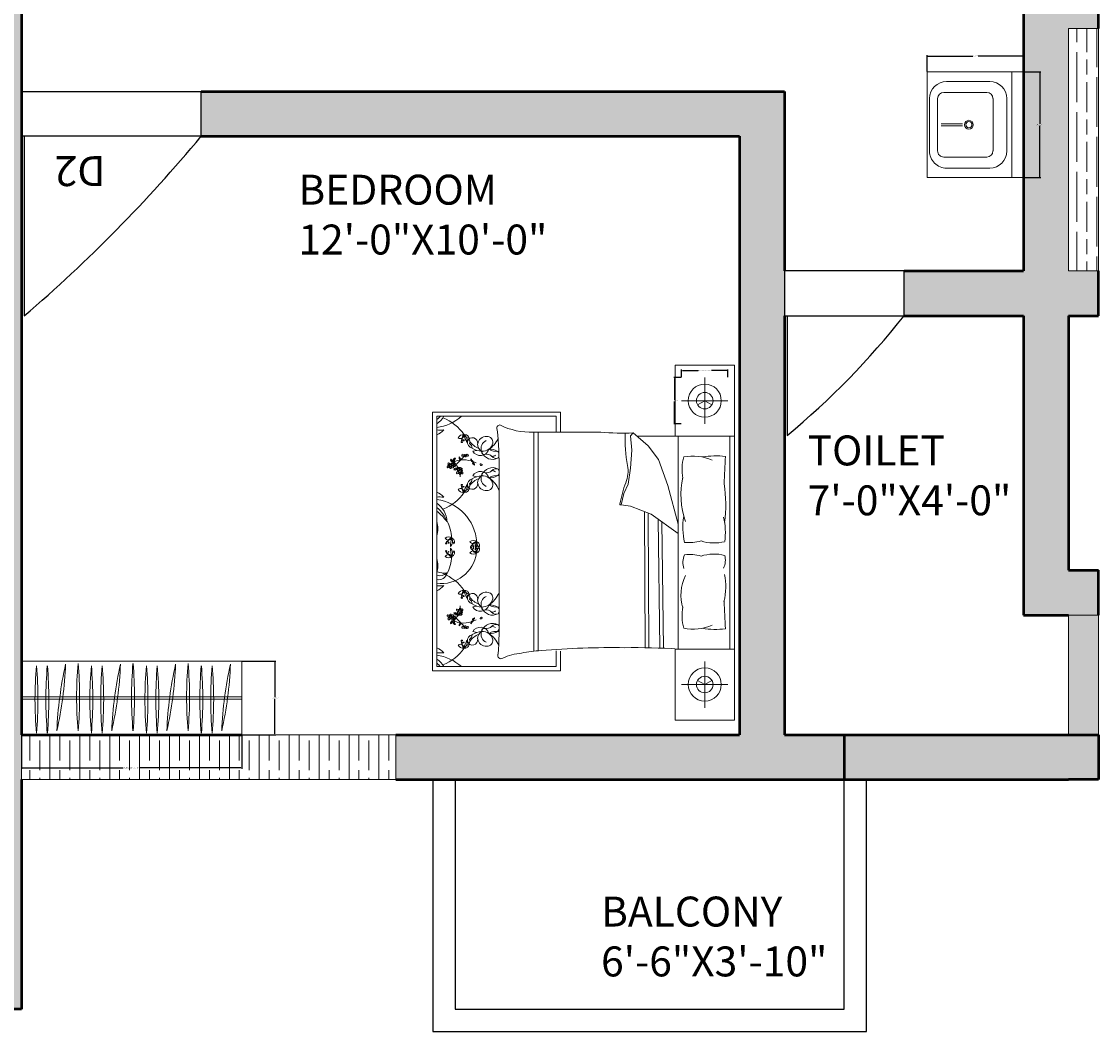
# Model space of a CAD drawing. Units: inches. Extents: x -12 to 604, y -566 to 58.
# Tile 3 of 12: x 388 to 604, y -534 to -332. Entities that reach past the tile are written whole.
import ezdxf

# ---------------------------------------------------------------- set-up
doc = ezdxf.new("R2010")
doc.units = ezdxf.units.IN
doc.header["$MEASUREMENT"] = 0
for name, color, linetype, lineweight in [('A-ANNO-DIMS', 2, 'Continuous', 18), ('A-ANNO-TEXT', 7, 'Continuous', 18), ('A-AREA-IDEN', 7, 'Continuous', 18), ('A-DOOR', 4, 'Continuous', 25), ('A-FLOR-FIXT', 9, 'Continuous', 18), ('A-FLOR-RAIL', 7, 'Continuous', 25), ('A-FURN', 8, 'Continuous', 18), ('A-GLAZ', 82, 'Continuous', 18), ('A-GLAZ-PATT', 82, 'Continuous', 13), ('A-WALL', 7, 'Continuous', 50), ('A-WALL-PATT', 18, 'Continuous', 13)]:
    doc.layers.add(name, color=color, linetype=linetype, lineweight=lineweight)
doc.styles.get("Standard").update_dxf_attribs({"font": 'arial.ttf'})
doc.dimstyles.get("Standard").update_dxf_attribs({"dimtxt": 0.18, "dimasz": 0.18, "dimexe": 0.18, "dimexo": 0.0625, "dimgap": 0.09, "dimtad": 0, "dimtih": 1, "dimtoh": 1, "dimdec": 0, "dimzin": 0, "dimdsep": 46, "dimlunit": 3, "dimtxsty": 'Standard', "dimcen": 0.09, "dimadec": 0, "dimazin": 0, "dimtfac": 1, "dimtdec": 0, "dimtofl": 0, "dimtmove": 0, "dimatfit": 3, "dimfxl": 1, "dimtolj": 1, "dimtzin": 0, "dimarcsym": 0})
pattern_1 = [(90, (0, 0), (6, -4e-16), [10, -2]), (90, (2, -2), (6, -4e-16), [6, -1.5, 3, -1.5]), (90, (4, -5), (6, -4e-16), [10, -2])]

# ---------------------------------------------------------------- blocks, each defined once
blk = doc.blocks.new('М14 600х655')
for p, q in [((-655, 600), (-655, 0)), ((-655, 600), (-655, 0)), ((-655, 0), (-655, 600)), ((0, 600), (-655, 600)), ((0, 0), (0, 600)), ((0, 525), (-655, 525)), ((-165.1, 494.1), (-489.9, 494.1)), ((-165.4, 408.4), (-490.2, 408.4)), ((-595.8, 388.1), (-595.8, 121.3)), ((-528.4, 370.1), (-528.4, 103.3)), ((-127.2, 103.3), (-127.2, 370.1)), ((-59.2, 121.3), (-59.2, 388.1)), ((-333.5, 87.1), (-333.5, 219.6)), ((-321.5, 87.1), (-321.5, 219.6)), ((-655, 0), (-655, 0)), ((-655, 0), (-655, 0)), ((-655, 0), (0, 0)), ((-655, 0), (0, 0)), ((-490.2, 65.1), (-165.4, 65.1)), ((-489.9, 15.4), (-165.1, 15.4))]:
    blk.add_line(p, q)
for radius in [27.6, 19.3]:
    blk.add_circle((-327.5, 258.9), radius)
for centre, radius, start, end in [((-489.9, 388.1), 105.9, 90, 180), ((-165.1, 388.1), 105.9, 0, 90), ((-490.2, 370.1), 38.2, 90, 180), ((-165.4, 370.1), 38.2, 0, 90), ((-489.9, 121.3), 105.9, 180, 270), ((-490.2, 103.3), 38.2, 180, 270), ((-165.4, 103.3), 38.2, 270, 0), ((-165.1, 121.3), 105.9, 270, 0)]:
    blk.add_arc(centre, radius, start, end)
blk = doc.blocks.new('WARDROBE-HANGING-RAIL')
for p, q in [((44.18, 14.73), (0, 14.73)), ((0, 14.73), (0, 0)), ((44.18, 14.73), (44.18, 0)), ((44.18, 7.61), (0, 7.61)), ((44.18, 7.12), (0, 7.12)), ((44.18, 0), (0, 0))]:
    blk.add_line(p, q)
for centre, start, end in [((80.19, 7.07), 175.0028, 184.9972), ((-74.2, 7.07), 355.0028, 4.9972), ((82.37, 7.07), 175.0028, 184.9972), ((-72.01, 7.07), 355.0028, 4.9972), ((-68.57, 17.55), 347.508, 357.5023), ((84.5, -2.59), 167.508, 177.5023), ((88.54, 7.54), 175.0028, 184.9972), ((-65.84, 7.54), 355.0028, 4.9972), ((91.2, 7.07), 175.0028, 184.9972), ((-63.19, 7.07), 355.0028, 4.9972), ((93.38, 7.07), 175.0028, 184.9972), ((-61.01, 7.07), 355.0028, 4.9972), ((-57.56, 17.55), 347.508, 357.5023), ((95.51, -2.59), 167.508, 177.5023), ((99.55, 7.54), 175.0028, 184.9972), ((-54.83, 7.54), 355.0028, 4.9972), ((102.24, 7.07), 175.0028, 184.9972), ((-52.14, 7.07), 355.0028, 4.9972), ((104.43, 7.07), 175.0028, 184.9972), ((-49.96, 7.07), 355.0028, 4.9972), ((106.56, -2.59), 167.508, 177.5023), ((-46.51, 17.55), 347.508, 357.5023), ((110.6, 7.54), 175.0028, 184.9972), ((-43.79, 7.54), 355.0028, 4.9972), ((113.25, 7.07), 175.0028, 184.9972), ((-41.13, 7.07), 355.0028, 4.9972), ((115.43, 7.07), 175.0028, 184.9972), ((-38.95, 7.07), 355.0028, 4.9972), ((117.56, -2.59), 167.508, 177.5023), ((-35.5, 17.55), 347.508, 357.5023)]:
    blk.add_arc(centre, 77.49, start, end)
blk = doc.blocks.new('BALCONY-RAIL-U')
for p, q in [((0, 50.5), (0, 4.5)), ((4.5, 50.5), (4.5, 4.5)), ((82.5, 4.5), (82.5, 50.5)), ((87, 4.5), (87, 50.5)), ((0, 4.5), (0, 0)), ((4.5, 4.5), (82.5, 4.5)), ((87, 0), (87, 4.5)), ((0, 0), (4.5, 0)), ((4.5, 0), (82.5, 0)), ((82.5, 0), (87, 0))]:
    blk.add_line(p, q)
blk = doc.blocks.new('BEDSIDE-LAMP-169')
for p, q in [((4.65, 9.3), (4.65, 0)), ((0, 4.65), (9.3, 4.65))]:
    blk.add_line(p, q)
for points in [[(4.65, 4.65), (3.21, 5.48)], [(4.65, 4.65), (6.09, 5.48)]]:
    blk.add_lwpolyline(points)
for radius in [3.32, 1.66]:
    blk.add_circle((4.65, 4.65), radius)
blk = doc.blocks.new('*D21')
at = {"layer": 'A-ANNO-DIMS', "color": 0, "lineweight": -2, "transparency": 16777216}
for p, q in [((388.32, -474.92), (388.32, -481.67)), ((432.5, -474.92), (432.5, -481.67)), ((388.5, -481.49), (408.68, -481.49)), ((432.32, -481.49), (412.15, -481.49))]:
    blk.add_line(p, q, dxfattribs=at)
at = {"layer": 'A-ANNO-DIMS', "color": 0, "transparency": 16777216}
for points in [[(388.5, -481.46), (388.5, -481.52), (388.32, -481.49)], [(432.32, -481.46), (432.32, -481.52), (432.5, -481.49)]]:
    blk.add_solid(points, dxfattribs=at)
at = {"layer": 'Defpoints', "color": 0, "transparency": 16777216}
for p in [(388.32, -474.86), (432.5, -474.86), (432.5, -481.49)]:
    blk.add_point(p, dxfattribs=at)
at = {"layer": 'A-ANNO-DIMS', "color": 0, "transparency": 16777216, "insert": (410.41, -481.49), "char_height": 0.18, "attachment_point": 5}
blk.add_mtext('\\A1;WARDROBE RAIL 3\'-8" TYP.', dxfattribs=at)
blk = doc.blocks.new('*D22')
at = {"layer": 'A-ANNO-DIMS', "color": 0, "lineweight": -2, "transparency": 16777216}
for p, q in [((432.57, -460.13), (439.31, -460.13)), ((439.13, -460.31), (439.13, -467.31)), ((439.13, -474.68), (439.13, -467.68)), ((432.57, -474.86), (439.31, -474.86))]:
    blk.add_line(p, q, dxfattribs=at)
at = {"layer": 'A-ANNO-DIMS', "color": 0, "transparency": 16777216}
for points in [[(439.1, -460.31), (439.16, -460.31), (439.13, -460.13)], [(439.1, -474.68), (439.16, -474.68), (439.13, -474.86)]]:
    blk.add_solid(points, dxfattribs=at)
at = {"layer": 'Defpoints', "color": 0, "transparency": 16777216}
for p in [(432.5, -460.13), (439.13, -460.13), (432.5, -474.86)]:
    blk.add_point(p, dxfattribs=at)
at = {"layer": 'A-ANNO-DIMS', "color": 0, "transparency": 16777216, "insert": (439.13, -467.5), "char_height": 0.18, "attachment_point": 5}
blk.add_mtext('\\A1;1\'-2 1/2" TYP.', dxfattribs=at)
blk = doc.blocks.new('*D25')
at = {"layer": 'A-ANNO-DIMS', "color": 0, "lineweight": -2, "transparency": 16777216}
for p, q in [((589.44, -341.95), (592.74, -341.95)), ((592.56, -342.13), (592.56, -352.37)), ((592.56, -362.98), (592.56, -352.74)), ((589.44, -363.16), (592.74, -363.16))]:
    blk.add_line(p, q, dxfattribs=at)
at = {"layer": 'A-ANNO-DIMS', "color": 0, "transparency": 16777216}
for points in [[(592.53, -342.13), (592.59, -342.13), (592.56, -341.95)], [(592.53, -362.98), (592.59, -362.98), (592.56, -363.16)]]:
    blk.add_solid(points, dxfattribs=at)
at = {"layer": 'Defpoints', "color": 0, "transparency": 16777216}
for p in [(589.38, -341.95), (589.38, -363.16), (592.56, -363.16)]:
    blk.add_point(p, dxfattribs=at)
at = {"layer": 'A-ANNO-DIMS', "color": 0, "transparency": 16777216, "insert": (592.56, -352.55), "char_height": 0.18, "attachment_point": 5}
blk.add_mtext('\\A1;BASIN 1\'-9"', dxfattribs=at)
blk = doc.blocks.new('*D26')
at = {"layer": 'A-ANNO-DIMS', "color": 0, "lineweight": -2, "transparency": 16777216}
for p, q in [((569.95, -341.89), (569.95, -338.59)), ((570.13, -338.77), (579.13, -338.77)), ((589.2, -338.77), (580.19, -338.77)), ((589.38, -341.89), (589.38, -338.59))]:
    blk.add_line(p, q, dxfattribs=at)
at = {"layer": 'A-ANNO-DIMS', "color": 0, "transparency": 16777216}
for points in [[(570.13, -338.74), (570.13, -338.8), (569.95, -338.77)], [(589.2, -338.74), (589.2, -338.8), (589.38, -338.77)]]:
    blk.add_solid(points, dxfattribs=at)
at = {"layer": 'Defpoints', "color": 0, "transparency": 16777216}
for p in [(589.38, -338.77), (569.95, -341.95), (589.38, -341.95)]:
    blk.add_point(p, dxfattribs=at)
at = {"layer": 'A-ANNO-DIMS', "color": 0, "transparency": 16777216, "insert": (579.66, -338.77), "char_height": 0.18, "attachment_point": 5}
blk.add_mtext('\\A1;1\'-7 1/2"', dxfattribs=at)
blk = doc.blocks.new('*D43')
at = {"layer": 'A-ANNO-DIMS', "color": 0, "lineweight": -2, "transparency": 16777216}
for p, q in [((520.71, -403.17), (520.71, -401.66)), ((530.01, -403.17), (530.01, -401.66)), ((520.89, -401.84), (524.01, -401.84)), ((529.83, -401.84), (526.71, -401.84))]:
    blk.add_line(p, q, dxfattribs=at)
at = {"layer": 'A-ANNO-DIMS', "color": 0, "transparency": 16777216}
for points in [[(520.89, -401.81), (520.89, -401.87), (520.71, -401.84)], [(529.83, -401.81), (529.83, -401.87), (530.01, -401.84)]]:
    blk.add_solid(points, dxfattribs=at)
at = {"layer": 'Defpoints', "color": 0, "transparency": 16777216}
for p in [(520.71, -401.84), (520.71, -403.23), (530.01, -403.23)]:
    blk.add_point(p, dxfattribs=at)
at = {"layer": 'A-ANNO-DIMS', "color": 0, "transparency": 16777216, "insert": (525.36, -401.84), "char_height": 0.18, "attachment_point": 5}
blk.add_mtext('\\A1;LAMP D 0\'-9 1/2" TYP.', dxfattribs=at)
blk = doc.blocks.new('*D44')
at = {"layer": 'A-ANNO-DIMS', "color": 0, "lineweight": -2, "transparency": 16777216}
for p, q in [((520.65, -403.23), (519.13, -403.23)), ((519.31, -403.41), (519.31, -407.7)), ((519.31, -412.35), (519.31, -408.06)), ((520.65, -412.53), (519.13, -412.53))]:
    blk.add_line(p, q, dxfattribs=at)
at = {"layer": 'A-ANNO-DIMS', "color": 0, "transparency": 16777216}
for points in [[(519.28, -403.41), (519.34, -403.41), (519.31, -403.23)], [(519.28, -412.35), (519.34, -412.35), (519.31, -412.53)]]:
    blk.add_solid(points, dxfattribs=at)
at = {"layer": 'Defpoints', "color": 0, "transparency": 16777216}
for p in [(520.71, -403.23), (519.31, -412.53), (520.71, -412.53)]:
    blk.add_point(p, dxfattribs=at)
at = {"layer": 'A-ANNO-DIMS', "color": 0, "transparency": 16777216, "insert": (519.31, -407.88), "char_height": 0.18, "attachment_point": 5}
blk.add_mtext('\\A1;0\'-9 1/2" TYP.', dxfattribs=at)

msp = doc.modelspace()

# ---------------------------------------------------------------- hatches: boundary and pattern name
at = {"layer": 'A-GLAZ-PATT'}
h = msp.add_hatch(dxfattribs=at)
h.set_pattern_fill('GOST_WOOD', color=256)
h.set_pattern_definition(pattern_1)
h.paths.add_polyline_path([(344.32, -529.86), (344.32, -520.86), (284.32, -520.86), (284.32, -529.86)])
h.paths.add_polyline_path([(604.32, -450.86), (598.32, -450.86), (598.32, -474.86), (604.32, -474.86)])
h.paths.add_polyline_path([(598.32, -309.28), (604.32, -309.28), (604.32, -274.86), (598.32, -274.86)])
h.paths.add_polyline_path([(598.32, -235.86), (604.32, -235.86), (604.32, -204.86), (598.32, -204.86)])
h.paths.add_polyline_path([(598.32, -159.86), (604.32, -159.86), (604.32, -99.86), (598.32, -99.86)])
h = msp.add_hatch(dxfattribs=at)
h.set_pattern_fill('GOST_WOOD', color=256)
h.set_pattern_definition(pattern_1)
h.paths.add_polyline_path([(604.32, -333.28), (598.32, -333.28), (598.32, -381.86), (604.32, -381.86)])
h = msp.add_hatch(dxfattribs=at)
h.set_pattern_fill('GOST_WOOD', color=256)
h.set_pattern_definition(pattern_1)
h.paths.add_polyline_path([(463.39, -474.86), (388.32, -474.86), (388.32, -483.86), (463.39, -483.86)])
at = {"layer": 'A-WALL-PATT'}
h = msp.add_hatch(color=256, dxfattribs=at)
h.dxf.hatch_style = 1
h.paths.add_polyline_path([(169.32, 11.14), (169.32, 17.14), (160.32, 17.14), (160.32, 11.14), (118.32, 11.14), (118.32, 6.64), (118.32, 2.14), (127.32, 2.14), (169.32, 2.14)])
h.paths.add_polyline_path([(127.32, -13.61), (118.32, -13.61), (118.32, -29.36), (34.82, -29.36), (24.32, -29.36), (24.32, -38.36), (39.32, -38.36), (118.32, -38.36), (118.32, -126.86), (127.32, -126.86), (127.32, -117.86)])
h.paths.add_polyline_path([(82.32, -92.36), (39.32, -92.36), (39.32, -56.22), (30.32, -56.22), (24.32, -56.22), (24.32, -65.22), (30.32, -65.22), (30.32, -113.36), (24.32, -113.36), (24.32, -122.36), (39.32, -122.36), (39.32, -101.36), (82.32, -101.36), (82.32, -96.86)], flags=17)
h.paths.add_polyline_path([(280.32, 11.14), (238.32, 11.14), (238.32, 17.14), (229.32, 17.14), (229.32, 12.64), (229.32, 11.14), (229.32, 2.14), (271.32, 2.14), (271.32, -117.86), (163.32, -117.86), (163.32, -126.86), (271.32, -126.86), (271.32, -189.86), (280.32, -189.86), (280.32, -180.86)])
h.paths.add_polyline_path([(415.32, 17.14), (406.32, 17.14), (406.32, 11.14), (358.32, 11.14), (358.32, -21.86), (367.32, -21.86), (367.32, 2.14), (415.32, 2.14)], flags=17)
h.paths.add_polyline_path([(484.55, -45.86), (448.32, -45.86), (448.32, 2.14), (448.32, 17.14), (439.32, 17.14), (439.32, 12.64), (439.32, 2.14), (439.32, -45.86), (367.32, -45.86), (358.32, -45.86), (358.32, -54.86), (430.32, -54.86), (430.32, -69.59), (430.32, -180.86), (318.82, -180.86), (318.82, -189.86), (318.82, -331.86), (327.82, -331.86), (327.82, -189.86), (439.32, -189.86), (439.32, -180.86), (439.32, -54.86), (483.5, -54.86), (484.55, -54.86)])
h.paths.add_polyline_path([(529.32, 11.14), (481.32, 11.14), (481.32, 17.14), (472.32, 17.14), (472.32, 12.64), (472.32, 2.14), (520.32, 2.14), (520.32, -21.86), (529.32, -21.86)])
h.paths.add_polyline_path([(598.32, -45.86), (582.42, -45.86), (582.42, -50.36), (582.42, -54.86), (589.32, -54.86), (589.32, -99.86), (598.32, -99.86), (604.32, -99.86), (604.32, -90.86), (598.32, -90.86)])
h.paths.add_polyline_path([(598.32, -168.86), (604.32, -168.86), (604.32, -159.86), (589.32, -159.86), (589.32, -180.86), (477.32, -180.86), (477.32, -189.86), (477.32, -259.86), (486.32, -259.86), (486.32, -189.86), (589.32, -189.86), (589.32, -204.86), (598.32, -204.86), (604.32, -204.86), (604.32, -195.86), (598.32, -195.86)])
h.paths.add_polyline_path([(598.32, -244.86), (604.32, -244.86), (604.32, -235.86), (598.32, -235.86), (589.32, -235.86), (589.32, -250.86), (522.32, -250.86), (522.32, -259.86), (589.32, -259.86), (589.32, -274.86), (598.32, -274.86), (604.32, -274.86), (604.32, -265.86), (598.32, -265.86)])
h.paths.add_polyline_path([(598.32, -333.28), (604.32, -333.28), (604.32, -324.28), (598.32, -324.28), (598.32, -321.87), (598.32, -318.28), (604.32, -318.28), (604.32, -309.28), (598.32, -309.28), (589.32, -309.28), (589.32, -341.95), (589.38, -341.95), (589.38, -363.16), (589.32, -381.86), (565.32, -381.86), (565.32, -390.86), (589.32, -390.86), (589.32, -450.86), (598.32, -450.86), (604.32, -450.86), (604.32, -441.86), (598.32, -441.86), (598.32, -390.86), (604.32, -390.86), (604.32, -381.86), (598.32, -381.86)])
h.paths.add_polyline_path([(541.32, -345.86), (424.32, -345.86), (424.32, -354.86), (532.32, -354.86), (532.32, -474.86), (463.39, -474.86), (463.39, -483.86), (553.32, -483.86), (553.32, -474.86), (541.32, -474.86), (541.32, -390.86), (541.32, -381.86)])
h.paths.add_polyline_path([(604.32, -474.86), (589.32, -474.86), (553.32, -474.86), (553.32, -483.86), (598.32, -483.86), (604.32, -483.86)])
h.paths.add_polyline_path([(388.32, -483.86), (388.32, -474.86), (388.32, -460.13), (388.32, -333.86), (388.32, -322.86), (379.32, -322.86), (379.32, -331.86), (379.32, -333.86), (379.32, -474.86), (379.32, -520.86), (344.32, -520.86), (344.32, -529.86), (379.32, -529.86), (388.32, -529.86)])
h.paths.add_polyline_path([(284.32, -520.86), (249.32, -520.86), (249.32, -474.86), (249.32, -368.36), (240.32, -368.36), (240.32, -474.86), (238.52, -474.86), (238.52, -483.86), (240.32, -483.86), (240.32, -529.86), (249.32, -529.86), (284.32, -529.86)])
h.paths.add_polyline_path([(178.82, -474.86), (158.91, -474.86), (158.91, -483.86), (162.32, -483.86), (178.82, -483.86)])
h.paths.add_polyline_path([(84.32, -474.86), (84.32, -366.86), (75.32, -366.86), (75.32, -474.86), (39.32, -474.86), (39.32, -453.86), (24.32, -453.86), (24.32, -462.86), (30.32, -462.86), (30.32, -483.86), (84.32, -483.86)])
h.paths.add_polyline_path([(39.32, -342.86), (75.32, -342.86), (84.32, -342.86), (179.67, -342.86), (179.67, -333.86), (39.32, -333.86), (39.32, -318.86), (24.32, -318.86), (24.32, -327.86), (30.32, -327.86), (30.32, -432.86), (24.32, -432.86), (24.32, -441.86), (30.32, -441.86), (39.32, -441.86)])
h.paths.add_polyline_path([(249.32, -252.86), (115.32, -252.86), (115.32, -225.86), (106.32, -225.86), (106.32, -252.86), (39.32, -252.86), (39.32, -237.86), (24.32, -237.86), (24.32, -246.86), (30.32, -246.86), (30.32, -267.86), (24.32, -267.86), (24.32, -276.86), (39.32, -276.86), (39.32, -261.86), (240.32, -261.86), (240.32, -331.86), (249.32, -331.86), (266.82, -331.86), (266.82, -322.86), (249.32, -322.86)])
h.paths.add_polyline_path([(127.32, -180.86), (39.32, -180.86), (24.32, -180.86), (24.32, -189.86), (39.32, -189.86), (127.32, -189.86)])
h.paths.add_polyline_path([(39.32, -159.86), (24.32, -159.86), (24.32, -168.86), (30.32, -168.86), (30.32, -180.86), (39.32, -180.86)])
h.paths.add_polyline_path([(470.51, -17.27), (512.48, -17.27), (512.48, 5.12), (470.51, 5.12)], flags=9)
h.paths.add_polyline_path([(484.21, -244.26), (526.45, -244.26), (526.45, -221.87), (484.21, -221.87)], flags=24)
h.paths.add_polyline_path([(36.91, -442.88), (83.54, -442.88), (83.54, -420.5), (36.91, -420.5)], flags=25)

# ---------------------------------------------------------------- linework, layer by layer
at = {"layer": 'A-DOOR'}
for p, q in [((388.32, -345.86), (388.32, -354.86)), ((388.32, -345.86), (424.32, -345.86)), ((424.32, -354.86), (424.32, -345.86)), ((424.32, -354.86), (388.32, -354.86)), ((388.87, -354.86), (388.87, -390.86)), ((541.32, -381.86), (541.32, -390.86)), ((565.32, -381.86), (541.32, -381.86)), ((565.32, -390.86), (565.32, -381.86)), ((541.32, -390.86), (565.32, -390.86)), ((541.87, -390.86), (541.87, -414.86))]:
    msp.add_line(p, q, dxfattribs=at)
for centre, radius, start, end in [((195.24, -164.69), 297.74, 310.567, 320.3026), ((441.72, -293.53), 157.32, 309.5397, 321.7836)]:
    msp.add_arc(centre, radius, start, end, dxfattribs=at)
at = {"layer": 'A-FURN'}
for p, q in [((531.29, -400.77), (531.29, -471.92)), ((470.78, -410.16), (496.41, -410.16)), ((470.78, -462.03), (470.78, -410.16)), ((496.41, -410.16), (496.41, -414.18)), ((471.6, -410.98), (471.6, -461.21)), ((495.58, -410.98), (471.6, -410.98)), ((495.58, -414.18), (495.58, -410.98)), ((491.08, -458.08), (491.08, -414.18)), ((491.97, -458.01), (491.97, -414.18)), ((510.44, -414.94), (511.02, -414.36)), ((511.02, -414.36), (514.04, -416.95)), ((510.73, -417.82), (510.44, -414.94)), ((531.29, -415), (511.76, -415)), ((520.04, -415), (520.04, -457.69)), ((530.37, -457.69), (530.37, -415)), ((478.82, -417.99), (479.62, -417.84)), ((510.44, -421.42), (510.73, -417.82)), ((514.04, -416.95), (516.06, -419.69)), ((516.06, -419.69), (517.93, -424.88)), ((478.82, -422.97), (479.62, -423.12)), ((484.09, -450.79), (484.09, -421.9)), ((510.01, -424.59), (510.44, -421.42)), ((509.14, -426.46), (510.01, -424.59)), ((517.93, -424.88), (520.04, -432.64)), ((508.57, -428.77), (509.14, -426.46)), ((510.44, -429.06), (508.57, -428.77)), ((514.62, -430.64), (510.44, -429.06)), ((513.39, -457.44), (513.27, -430.13)), ((514.12, -457.43), (514.01, -430.41)), ((520.04, -434.54), (514.62, -430.64)), ((516.36, -457.47), (515.99, -431.63)), ((517.09, -457.5), (516.73, -432.16)), ((478.82, -449.22), (479.62, -449.06)), ((478.82, -454.19), (479.62, -454.35)), ((495.58, -461.21), (495.58, -458.07)), ((496.41, -458.08), (496.41, -462.03)), ((496.41, -462.03), (470.78, -462.03)), ((471.6, -461.21), (495.58, -461.21))]:
    msp.add_line(p, q, dxfattribs=at)
for points in [[(519.43, -415), (519.43, -400.77), (531.29, -400.77)], [(531.29, -457.69), (519.43, -457.69), (519.43, -471.92), (531.29, -471.92)]]:
    msp.add_lwpolyline(points, dxfattribs=at)
for points in [[(504.5, -414.21, 0.001242), (491, -414.18, -0.127202), (484.27, -412.75)], [(529.51, -419.08, 0.074897), (524.87, -419.17, -0.472817)], [(524.61, -436.01, 0.14099), (529.35, -436.15, 0.235245)], [(524.61, -439.05, -0.14099), (529.35, -438.9, -0.235245)], [(529.51, -453.6, -0.074897), (524.87, -453.51, 0.472817)], [(492.53, -457.99, 0.056112), (488.62, -458.51, 0.095341), (484.85, -459.51)]]:
    msp.add_lwpolyline(points, format="xyb", dxfattribs=at)
for centre in [(474.33, -420.92), (476.24, -422.1), (474.33, -451.27), (476.24, -450.08)]:
    msp.add_circle(centre, 0.181, dxfattribs=at)
for centre, radius, start, end in [((468.26, -407.1), 5.64, 306.3036, 316.4814), ((469.11, -408.73), 4.53, 303.4617, 330.1116), ((470.35, -404.06), 9.29, 277.745, 311.8856), ((469.43, -419.96), 9.29, 34.3865, 68.5908), ((470.15, -411.26), 3.78, 292.5547, 318.9546), ((472.18, -400.91), 12.86, 267.4081, 273.6519), ((476.88, -415.72), 1.03, 77.7115, 159.0387), ((476.32, -414.69), 0.776, 238.4633, 358.2869), ((478.87, -416.26), 2.35, 138.8402, 177.9352), ((477.45, -415.39), 0.76, 117.6827, 223.7762), ((477.28, -415.46), 0.77, 2.9516, 103.728), ((483.44, -413.3), 6.5, 192.5173, 207.1824), ((476.24, -415.9), 1.47, 345.4653, 54.2343), ((478.45, -413.89), 1.59, 211.3827, 255.2969), ((484.32, -413.4), 0.657, 93.98, 207.3412), ((410.03, -421.05), 74.07, 359.3433, 5.6887), ((509.25, -349.12), 65.26, 265.8294, 271.553), ((536.21, -415.58), 26.85, 177.4519, 191.3392), ((476.63, -416.18), 0.115, 177.9352, 11.4834), ((476.69, -416.17), 0.0561, 11.4834, 127.9409), ((476.98, -415.84), 0.101, 223.7762, 159.7183), ((478.76, -416.37), 1.07, 350.264, 160.8688), ((479.08, -416.11), 1.33, 175.969, 254.3045), ((477.6, -416.15), 0.654, 333.9755, 53.2681), ((477.31, -417.55), 1.42, 6.1662, 51.5825), ((481.11, -414.25), 3.36, 211.2614, 251.7045), ((481.5, -416.76), 1.7, 84.9449, 172.8857), ((481.87, -416.46), 2.07, 182.3591, 234.0401), ((482.14, -417.43), 1.65, 111.5819, 201.4221), ((480.78, -415.9), 2.14, 265.2933, 346.921), ((481.67, -416.26), 1.2, 354.4856, 91.0538), ((479.08, -413.13), 5.39, 303.6671, 333.2997), ((471.83, -414.81), 6.76, 313.1541, 322.0459), ((476.79, -418.87), 0.139, 142.4737, 265.053), ((476.98, -418.84), 0.299, 127.7621, 169.0403), ((476.82, -418.58), 0.421, 265.053, 338.3618), ((477.38, -419.16), 0.55, 113.4276, 137.6104), ((477.31, -418.59), 0.181, 183.2768, 356.7232), ((477.45, -418.92), 0.297, 139.7889, 227.6792), ((476.75, -418.92), 0.593, 353.0852, 15.7171), ((477.14, -418.99), 0.375, 350.3487, 43.6538), ((477.83, -418.6), 0.436, 198.7263, 262.5032), ((477.49, -418.8), 0.173, 1.1081, 91.8675), ((477.81, -418.9), 0.14, 255.2356, 54.9248), ((477.59, -418.84), 0.302, 11.5637, 52.6358), ((480.84, -414.22), 3.82, 236.2883, 266.5076), ((480.35, -417.11), 1.77, 209.9085, 343.1337), ((481.09, -418.23), 0.442, 167.3041, 285.1471), ((482.29, -420.34), 2.74, 122.7011, 126.3445), ((482.8, -417.39), 2.27, 199.2822, 299.1751), ((481.59, -420.07), 1.46, 41.5653, 105.1471), ((483.57, -415.1), 2.95, 238.8218, 279.1554), ((482.29, -420.34), 2.74, 55.785, 94.7304), ((482.39, -417.04), 2.05, 277.436, 299.9149), ((483.31, -418.75), 0.857, 30.0293, 52.325), ((523, -428.15), 9.17, 65.1316, 101.7583), ((473.81, -421.19), 0.139, 142.4737, 265.053), ((473.99, -421.17), 0.299, 61.2196, 169.0403), ((473.83, -420.91), 0.421, 265.053, 338.3618), ((474.19, -420.55), 0.358, 157.4086, 261.4386), ((473.99, -420.54), 0.18, 58.0499, 135.6268), ((474.39, -421.49), 0.55, 113.4276, 137.6104), ((474.17, -420.65), 0.12, 172.906, 277.132), ((473.78, -420.87), 0.571, 14.7558, 58.0499), ((474.46, -421.25), 0.297, 139.7889, 227.6792), ((474.58, -420.72), 0.247, 36.1046, 181.4281), ((473.76, -421.24), 0.593, 353.0852, 15.7171), ((474.59, -419.75), 0.202, 124.3538, 214.3923), ((474.89, -419.78), 0.472, 190.3057, 287.1958), ((474.15, -421.31), 0.375, 350.3487, 43.6538), ((474.84, -420.93), 0.436, 198.7263, 262.5032), ((474.44, -420.52), 0.249, 270.0645, 331.1507), ((474.65, -420.58), 0.285, 221.8413, 265.7877), ((475.02, -419.61), 0.548, 176.9701, 248.2913), ((478.93, -416.72), 5.29, 212.6784, 216.3746), ((474.5, -421.13), 0.173, 1.1081, 91.8675), ((474.65, -420.69), 0.178, 263.7526, 41.7054), ((474.61, -421.17), 0.302, 11.5637, 86.365), ((474.84, -419.74), 0.209, 216.3746, 291.7548), ((476.69, -422.68), 2.95, 124.0033, 132.4917), ((474.82, -421.22), 0.14, 255.2356, 54.9248), ((473.65, -423.05), 3.16, 63.7819, 68.2913), ((475.34, -420.62), 0.502, 128.3208, 208.8162), ((475.34, -419.89), 0.472, 122.8155, 187.3992), ((475.43, -420.59), 0.6, 207.7043, 254.3516), ((474.98, -420.08), 0.158, 289.3605, 111.7548), ((475.09, -420.08), 0.158, 221.8703, 44.2646), ((475.81, -420.54), 0.826, 157.2305, 229.0635), ((475.55, -419.95), 0.548, 109.4799, 177.6828), ((475.04, -420.93), 0.826, 270.278, 342.111), ((475.53, -420.27), 0.486, 174.4544, 220.6188), ((472.77, -422.98), 3.54, 30.544, 49.818), ((475.25, -419.6), 0.202, 56.8636, 146.9021), ((475.36, -419.83), 0.209, 148.8844, 224.2646), ((474.72, -420.97), 0.584, 340.0041, 40.6188), ((479.71, -422.45), 5.29, 145.1882, 148.8844), ((476.69, -422.68), 2.95, 94.756, 119.2041), ((482.98, -426.93), 9.72, 132.2412, 142.1744), ((475.43, -420.91), 0.486, 278.7227, 324.8872), ((476.32, -421.16), 0.502, 182.8499, 266.1226), ((476.13, -420.8), 0.486, 231.7607, 277.9252), ((476.51, -420.72), 0.826, 214.5369, 286.3699), ((478.08, -419.2), 2.01, 178.3264, 187.1302), ((475.91, -419.47), 0.374, 11.3256, 64.4621), ((477.18, -418.94), 1.12, 190.2588, 210.656), ((476.42, -419.4), 0.341, 188.3432, 274.2869), ((476.72, -419.21), 0.596, 210.656, 242.6341), ((477.17, -418.69), 1.14, 218.2101, 226.3071), ((476.33, -419.65), 0.145, 325.7657, 67.4417), ((476.84, -425.62), 5.89, 73.5842, 93.8277), ((477.35, -419.02), 0.156, 227.6792, 350.3487), ((480.47, -419.62), 2.01, 178.3264, 187.1302), ((478.3, -419.9), 0.374, 11.3256, 64.4621), ((479.57, -419.36), 1.12, 190.2588, 210.656), ((478.82, -419.82), 0.341, 188.3432, 274.2869), ((479.12, -419.63), 0.596, 210.656, 242.6341), ((479.57, -419.12), 1.14, 218.2101, 226.3071), ((478.72, -420.08), 0.145, 325.7657, 67.4417), ((479.13, -420.34), 0.341, 147.5332, 233.4768), ((479.44, -420.17), 0.596, 179.1859, 211.164), ((478.86, -420.3), 0.145, 354.3784, 96.0543), ((476.84, -425.62), 5.89, 63.0032, 69.8941), ((479.89, -419.89), 1.12, 211.164, 231.5612), ((480.09, -418.98), 2.01, 234.6898, 243.4936), ((480.1, -420.01), 1.14, 195.5129, 203.6099), ((478.82, -420.76), 0.374, 357.3579, 50.4944), ((480.42, -420.68), 0.137, 12.7051, 190.4384), ((480.51, -420.67), 0.223, 190.4384, 10.4136), ((483.48, -418.39), 1.06, 221.5653, 293.8354), ((483.31, -418.75), 0.857, 314.4517, 333.558), ((504.2, -422), 5.79, 336.2616, 11.3392), ((530.35, -421.62), 9.54, 165.1039, 191.0369), ((1206.65, -458.3), 678.27, 176.68521, 177.14978), ((474.37, -421.35), 0.156, 227.6792, 350.3487), ((475.59, -421.96), 0.584, 98.7227, 159.3375), ((475.3, -421.21), 0.6, 244.9899, 291.6373), ((475.34, -421.3), 0.502, 290.5253, 358.5375), ((475.72, -422.38), 0.139, 142.4737, 265.053), ((475.9, -422.35), 0.299, 61.2196, 169.0403), ((475.74, -422.1), 0.421, 265.053, 338.3618), ((476.1, -421.74), 0.358, 157.4086, 261.4386), ((475.9, -421.72), 0.18, 58.0499, 135.6268), ((476.3, -422.67), 0.55, 113.4276, 137.6104), ((476.08, -421.84), 0.12, 172.906, 277.132), ((475.69, -422.06), 0.571, 14.7558, 58.0499), ((472.77, -422.98), 3.54, 23.0501, 23.8477), ((476.37, -422.43), 0.297, 139.7889, 227.6792), ((476.28, -422.54), 0.156, 227.6792, 350.3487), ((476.27, -421.86), 0.584, 37.3105, 97.9252), ((476.49, -421.9), 0.247, 36.1046, 181.4281), ((475.67, -422.43), 0.593, 353.0852, 15.7171), ((476.34, -421.06), 0.6, 265.0106, 311.658), ((472.77, -422.98), 3.54, 357.1071, 4.7585), ((476.06, -422.5), 0.375, 350.3487, 43.6538), ((476.75, -422.11), 0.436, 198.7263, 262.5032), ((476.35, -421.71), 0.249, 270.0645, 331.1507), ((476.56, -421.77), 0.285, 221.8413, 265.7877), ((476.41, -422.32), 0.173, 1.1081, 91.8675), ((476.56, -421.88), 0.178, 263.7526, 41.7054), ((476.52, -422.35), 0.302, 11.5637, 86.365), ((476.73, -422.41), 0.14, 255.2356, 54.9248), ((480.84, -426.74), 3.82, 93.4924, 123.7117), ((480.35, -423.85), 1.77, 16.8663, 150.0915), ((481.87, -424.5), 2.07, 125.9599, 177.6409), ((482.14, -423.53), 1.65, 158.5779, 248.4181), ((480.78, -425.06), 2.14, 13.079, 94.7067), ((481.09, -422.73), 0.442, 74.8529, 192.6959), ((482.8, -423.57), 2.27, 60.8249, 160.7178), ((482.29, -420.61), 2.74, 233.6555, 237.2989), ((481.59, -420.89), 1.46, 254.8529, 318.4347), ((483.57, -425.86), 2.95, 79.7133, 121.1782), ((482.29, -420.61), 2.74, 265.2696, 304.215), ((479.08, -427.83), 5.39, 21.4941, 56.3329), ((482.39, -423.92), 2.05, 60.0851, 82.564), ((483.48, -422.57), 1.06, 66.1646, 138.4347), ((483.31, -422.21), 0.857, 307.675, 336.7144), ((483.31, -422.21), 0.857, 23.229, 45.5483), ((537.12, -426.64), 16.54, 168.0397, 199.2615), ((476.32, -426.27), 0.776, 1.7131, 121.5367), ((476.63, -424.78), 0.115, 348.5166, 182.0648), ((478.87, -424.7), 2.35, 182.0648, 221.1598), ((476.69, -424.79), 0.0561, 232.0591, 348.5166), ((477.45, -425.57), 0.76, 136.2238, 242.3173), ((477.01, -425.13), 0.0606, 200.2667, 136.2271), ((476.24, -425.05), 1.47, 305.7657, 14.5347), ((483.44, -427.66), 6.5, 152.8176, 167.4827), ((479.08, -424.85), 1.33, 105.6955, 184.031), ((478.76, -424.59), 1.07, 199.1312, 9.736), ((477.6, -424.81), 0.654, 306.7319, 26.0245), ((477.31, -423.41), 1.42, 308.4175, 353.8338), ((481.11, -426.71), 3.36, 108.2955, 148.7386), ((481.5, -424.2), 1.7, 187.1143, 275.0551), ((481.67, -424.69), 1.2, 268.9462, 5.5144), ((535.45, -433.71), 27.59, 160.1194, 169.3383), ((503.77, -428.83), 25.81, 352.2196, 9.497), ((470.15, -429.7), 3.78, 41.0454, 67.4453), ((472.18, -440.05), 12.86, 86.3481, 92.5919), ((469.43, -421), 9.29, 291.4092, 325.6135), ((476.88, -425.24), 1.03, 200.9613, 282.2885), ((477.28, -425.5), 0.77, 256.272, 357.0484), ((478.45, -427.07), 1.59, 104.7031, 148.6173), ((470.35, -436.9), 9.29, 4.4623, 82.255), ((469.11, -432.23), 4.53, 1.272, 56.5383), ((468.26, -433.86), 5.64, 17.8504, 53.6964), ((508.51, -428.61), 0.172, 178.8623, 289.7536), ((466.67, -436.83), 8.39, 34.0123, 54.053), ((465.37, -436.18), 9.29, 4.4623, 27.4146), ((533.51, -433.34), 12.55, 169.8617, 193.6238), ((516.81, -434.28), 12.68, 351.5249, 13.96), ((466.72, -433.59), 5.11, 343.5431, 17.0202), ((464.08, -435.61), 7.55, 4.3787, 5.6357), ((458.91, -439.59), 13.5, 19.7217, 19.9028), ((473.94, -436.22), 1.03, 47.7873, 129.1145), ((473.98, -435.05), 0.776, 208.5391, 328.3627), ((475.4, -437.68), 2.35, 108.9159, 148.011), ((474.61, -436.22), 0.76, 87.7585, 193.852), ((473.97, -436.38), 0.101, 193.852, 129.9245), ((480.84, -437.41), 6.5, 162.593, 177.2582), ((473.3, -436.07), 1.47, 315.5411, 24.3101), ((476.22, -435.42), 1.59, 181.4585, 225.3727), ((474.42, -436.2), 0.77, 333.0274, 73.8037), ((478.92, -436.94), 1.03, 47.7873, 129.1145), ((478.95, -435.77), 0.776, 208.5391, 328.3627), ((480.37, -438.4), 2.35, 108.9159, 148.011), ((479.58, -436.93), 0.76, 87.7585, 193.852), ((478.27, -436.78), 1.47, 315.5411, 24.3101), ((485.82, -438.12), 6.5, 162.593, 177.2582), ((479.4, -436.91), 0.77, 333.0274, 73.8037), ((481.2, -436.13), 1.59, 181.4585, 225.3727), ((522.23, -427.62), 8.72, 264.0129, 285.8293), ((472.49, -437.36), 7.19, 262.8636, 351.8197), ((473.5, -436.5), 0.115, 148.011, 341.5592), ((473.5, -438.06), 0.115, 18.4408, 211.989), ((475.4, -436.88), 2.35, 211.989, 251.0841), ((473.56, -436.52), 0.0561, 341.5592, 98.0167), ((473.56, -438.04), 0.0561, 261.9833, 18.4408), ((474.61, -438.34), 0.76, 166.148, 272.2415), ((474, -438.17), 0.0606, 230.1909, 166.0209), ((480.84, -437.15), 6.5, 182.7418, 197.407), ((473.3, -438.49), 1.47, 335.6899, 44.4589), ((476.22, -439.14), 1.59, 134.6273, 178.5415), ((474.42, -438.36), 0.77, 286.1963, 26.9726), ((478.95, -438.79), 0.776, 31.6373, 151.4609), ((478.92, -437.62), 1.03, 230.8855, 312.2127), ((478.48, -437.21), 0.115, 148.011, 341.5592), ((478.48, -437.35), 0.115, 18.4408, 211.989), ((480.37, -436.16), 2.35, 211.989, 251.0841), ((478.54, -437.23), 0.0561, 341.5592, 98.0167), ((478.54, -437.33), 0.0561, 261.9833, 18.4408), ((479.58, -437.63), 0.76, 166.148, 272.2415), ((478.94, -437.09), 0.101, 193.852, 129.9245), ((478.98, -437.46), 0.0606, 230.1909, 166.0209), ((478.27, -437.78), 1.47, 335.6899, 44.4589), ((485.82, -436.44), 6.5, 182.7418, 197.407), ((479.4, -437.65), 0.77, 286.1963, 26.9726), ((481.2, -438.43), 1.59, 134.6273, 178.5415), ((466.72, -440.97), 5.11, 342.9798, 16.4569), ((464.08, -438.95), 7.55, 354.3643, 355.6213), ((458.91, -434.97), 13.5, 340.0972, 340.2783), ((473.98, -439.51), 0.776, 31.6373, 151.4609), ((473.94, -438.34), 1.03, 230.8855, 312.2127), ((465.37, -438.38), 9.29, 332.5854, 355.5377), ((524.74, -440.36), 3.77, 155.0183, 198.5407), ((522.23, -447.43), 8.72, 74.1707, 95.9871), ((525.97, -439.88), 3.52, 333.3437, 16.1026), ((473.15, -438.29), 4.16, 248.117, 276.6195), ((471.99, -442.11), 1.67, 256.3898, 349.0739), ((472.22, -440.86), 2.11, 252.8609, 311.9049), ((469.43, -451.19), 9.29, 34.3865, 68.5908), ((517.06, -445.16), 12.51, 346.3427, 11.1841), ((529.64, -446.95), 9.06, 153.8761, 196.1746), ((472.18, -432.14), 12.86, 267.4081, 273.6519), ((470.15, -442.49), 3.78, 292.5547, 318.9546), ((476.88, -446.95), 1.03, 77.7115, 159.0387), ((476.32, -445.92), 0.776, 238.4633, 358.2869), ((478.87, -447.49), 2.35, 138.8402, 177.9352), ((477.45, -446.61), 0.76, 117.6827, 223.7762), ((476.98, -447.07), 0.101, 223.7762, 159.7183), ((477.28, -446.69), 0.77, 2.9516, 103.728), ((478.45, -445.11), 1.59, 211.3827, 255.2969), ((476.24, -447.13), 1.47, 345.4653, 54.2343), ((483.44, -444.53), 6.5, 192.5173, 207.1824), ((478.76, -447.59), 1.07, 350.264, 160.8688), ((477.6, -447.37), 0.654, 333.9755, 53.2681), ((481.5, -447.98), 1.7, 84.9449, 172.8857), ((482.14, -448.65), 1.65, 111.5819, 201.4221), ((481.67, -447.49), 1.2, 354.4856, 91.0538), ((479.08, -444.36), 5.39, 303.6671, 338.5059), ((472.77, -449.2), 3.54, 355.2415, 2.8929), ((476.63, -447.41), 0.115, 177.9352, 11.4834), ((476.69, -447.4), 0.0561, 11.4834, 127.9409), ((479.08, -447.34), 1.33, 175.969, 254.3045), ((477.31, -448.77), 1.42, 6.1662, 51.5825), ((481.11, -445.48), 3.36, 211.2614, 251.7045), ((480.84, -445.45), 3.82, 236.2883, 266.5076), ((480.35, -448.34), 1.77, 209.9085, 343.1337), ((481.87, -447.69), 2.07, 182.3591, 234.0401), ((480.78, -447.12), 2.14, 265.2933, 346.921), ((482.29, -451.57), 2.74, 122.7011, 126.3445), ((483.57, -446.33), 2.95, 238.8218, 280.2867), ((482.29, -451.57), 2.74, 55.785, 94.7304), ((530.35, -451.06), 9.54, 168.9631, 194.8961), ((1206.65, -414.38), 678.27, 182.85022, 183.31479), ((473.81, -450.99), 0.139, 94.947, 217.5263), ((473.99, -451.02), 0.299, 190.9597, 298.7804), ((473.83, -451.27), 0.421, 21.6382, 94.947), ((474.19, -451.64), 0.358, 98.5614, 202.5914), ((474.39, -450.7), 0.55, 222.3896, 246.5724), ((474.17, -451.54), 0.12, 82.868, 187.094), ((474.46, -450.94), 0.297, 132.3208, 220.2111), ((474.37, -450.84), 0.156, 9.6513, 132.3208), ((473.76, -450.94), 0.593, 344.2829, 6.9148), ((474.15, -450.87), 0.375, 316.3462, 9.6513), ((474.84, -451.26), 0.436, 97.4968, 161.2737), ((474.65, -451.6), 0.285, 94.2123, 138.1587), ((474.44, -451.66), 0.249, 28.8493, 89.9355), ((474.5, -451.06), 0.173, 268.1325, 358.8919), ((474.61, -451.02), 0.302, 273.635, 348.4363), ((474.65, -451.5), 0.178, 318.2946, 96.2474), ((474.82, -450.96), 0.14, 305.0752, 104.7644), ((475.34, -451.56), 0.502, 151.1838, 231.6792), ((475.43, -451.6), 0.6, 105.6484, 152.2957), ((475.81, -451.65), 0.826, 130.9365, 202.7695), ((475.3, -450.97), 0.6, 68.3627, 115.0101), ((475.04, -451.26), 0.826, 17.889, 89.722), ((475.59, -450.22), 0.584, 200.6625, 261.2773), ((472.77, -449.2), 3.54, 310.182, 329.456), ((474.72, -451.22), 0.584, 319.3812, 19.9959), ((482.98, -445.25), 9.72, 217.8256, 227.7588), ((475.43, -451.28), 0.486, 35.1128, 81.2773), ((475.34, -450.89), 0.502, 1.4625, 69.4747), ((475.72, -449.81), 0.139, 94.947, 217.5263), ((475.9, -449.84), 0.299, 190.9597, 298.7804), ((475.74, -450.09), 0.421, 21.6382, 94.947), ((476.1, -450.45), 0.358, 98.5614, 202.5914), ((475.9, -450.46), 0.18, 224.3732, 301.9501), ((476.32, -451.03), 0.502, 93.8774, 177.1501), ((476.51, -451.47), 0.826, 73.6301, 145.4631), ((476.13, -451.38), 0.486, 82.0748, 128.2393), ((476.3, -449.51), 0.55, 222.3896, 246.5724), ((476.08, -450.35), 0.12, 82.868, 187.094), ((475.69, -450.13), 0.571, 301.9501, 345.2442), ((472.77, -449.2), 3.54, 336.1523, 336.9499), ((476.37, -449.76), 0.297, 132.3208, 220.2111), ((476.28, -449.65), 0.156, 9.6513, 132.3208), ((476.27, -450.32), 0.584, 262.0748, 322.6895), ((475.67, -449.76), 0.593, 344.2829, 6.9148), ((476.49, -450.28), 0.247, 178.5719, 323.8954), ((476.34, -451.13), 0.6, 48.342, 94.9894), ((476.06, -449.69), 0.375, 316.3462, 9.6513), ((476.75, -450.08), 0.436, 97.4968, 161.2737), ((476.56, -450.42), 0.285, 94.2123, 138.1587), ((476.35, -450.48), 0.249, 28.8493, 89.9355), ((476.41, -449.87), 0.173, 268.1325, 358.8919), ((476.52, -449.83), 0.302, 273.635, 348.4363), ((476.56, -450.31), 0.178, 318.2946, 96.2474), ((476.73, -449.78), 0.14, 305.0752, 104.7644), ((479.89, -452.29), 1.12, 128.4388, 148.836), ((480.09, -453.21), 2.01, 116.5064, 125.3102), ((478.82, -451.43), 0.374, 309.5056, 2.6421), ((480.51, -451.52), 0.223, 349.5864, 169.5616), ((481.09, -449.46), 0.442, 167.3041, 285.1471), ((482.8, -448.61), 2.27, 199.2822, 299.1751), ((481.59, -451.29), 1.46, 41.5653, 105.1471), ((482.39, -448.27), 2.05, 277.436, 299.9149), ((483.48, -449.62), 1.06, 221.5653, 293.8354), ((483.31, -449.98), 0.857, 23.2856, 52.325), ((414.89, -452.97), 69.24, 355.2402, 1.8035), ((483.31, -449.98), 0.857, 314.4517, 336.7144), ((473.99, -451.65), 0.18, 224.3732, 301.9501), ((473.78, -451.32), 0.571, 301.9501, 345.2442), ((474.58, -451.47), 0.247, 178.5719, 323.8954), ((474.59, -452.44), 0.202, 145.6077, 235.6462), ((474.89, -452.41), 0.472, 72.8042, 169.6943), ((475.02, -452.58), 0.548, 111.7087, 183.0299), ((478.93, -455.46), 5.29, 143.6254, 147.3216), ((474.84, -452.45), 0.209, 68.2452, 143.6254), ((476.69, -449.51), 2.95, 227.5083, 235.9967), ((473.65, -449.13), 3.16, 291.7087, 296.2181), ((475.34, -452.3), 0.472, 172.6008, 237.1845), ((474.98, -452.11), 0.158, 248.2452, 70.6395), ((475.09, -452.11), 0.158, 315.7354, 138.1297), ((475.55, -452.24), 0.548, 182.3172, 250.5201), ((475.53, -451.92), 0.486, 139.3812, 185.5456), ((475.25, -452.59), 0.202, 213.0979, 303.1364), ((475.36, -452.36), 0.209, 135.7354, 211.1156), ((479.71, -449.73), 5.29, 211.1156, 214.8118), ((476.69, -449.51), 2.95, 240.7959, 265.244), ((477.18, -453.25), 1.12, 149.344, 169.7412), ((478.08, -452.99), 2.01, 172.8698, 181.6736), ((475.91, -452.71), 0.374, 295.5379, 348.6744), ((476.42, -452.79), 0.341, 85.7131, 171.6568), ((476.72, -452.98), 0.596, 117.3659, 149.344), ((477.17, -453.49), 1.14, 133.6929, 141.7899), ((476.33, -452.53), 0.145, 292.5583, 34.2343), ((476.84, -446.57), 5.89, 266.1723, 286.4158), ((471.83, -457.38), 6.76, 37.9541, 46.8459), ((476.79, -453.32), 0.139, 94.947, 217.5263), ((476.98, -453.35), 0.299, 190.9597, 232.2379), ((476.82, -453.6), 0.421, 21.6382, 94.947), ((477.38, -453.03), 0.55, 222.3896, 246.5724), ((477.31, -453.6), 0.181, 3.2768, 176.7232), ((477.45, -453.27), 0.297, 132.3208, 220.2111), ((477.35, -453.16), 0.156, 9.6513, 132.3208), ((476.75, -453.27), 0.593, 344.2829, 6.9148), ((477.14, -453.2), 0.375, 316.3462, 9.6513), ((477.83, -453.59), 0.436, 97.4968, 161.2737), ((477.49, -453.38), 0.173, 268.1325, 358.8919), ((477.81, -453.29), 0.14, 305.0752, 104.7644), ((477.59, -453.35), 0.302, 307.3642, 348.4363), ((479.57, -452.83), 1.12, 149.344, 169.7412), ((480.47, -452.57), 2.01, 172.8698, 181.6736), ((478.3, -452.29), 0.374, 295.5379, 348.6744), ((478.82, -452.37), 0.341, 85.7131, 171.6568), ((479.12, -452.56), 0.596, 117.3659, 149.344), ((479.57, -453.07), 1.14, 133.6929, 141.7899), ((478.72, -452.11), 0.145, 292.5583, 34.2343), ((479.13, -451.84), 0.341, 126.5232, 212.4668), ((480.35, -455.08), 1.77, 16.8663, 150.0915), ((479.44, -452.02), 0.596, 148.836, 180.8141), ((478.86, -451.88), 0.145, 263.9457, 5.6216), ((476.84, -446.57), 5.89, 290.1059, 296.9968), ((480.1, -452.17), 1.14, 156.3901, 164.4871), ((480.42, -451.5), 0.137, 169.5616, 347.2949), ((481.09, -453.96), 0.442, 74.8529, 192.6959), ((482.8, -454.8), 2.27, 60.8249, 160.7178), ((481.59, -452.12), 1.46, 254.8529, 318.4347), ((482.39, -455.14), 2.05, 60.0851, 82.564), ((483.48, -453.8), 1.06, 66.1646, 138.4347), ((483.31, -453.43), 0.857, 16.6343, 45.5483), ((523, -444.54), 9.17, 258.2417, 294.8684), ((479.08, -456.08), 1.33, 105.6955, 184.031), ((478.76, -455.82), 1.07, 199.1312, 9.736), ((477.6, -456.04), 0.654, 306.7319, 26.0245), ((477.31, -454.64), 1.42, 308.4175, 353.8338), ((481.11, -457.94), 3.36, 108.2955, 148.7386), ((480.84, -457.97), 3.82, 93.4924, 123.7117), ((481.87, -455.73), 2.07, 125.9599, 177.6409), ((481.5, -455.43), 1.7, 187.1143, 275.0551), ((482.14, -454.76), 1.65, 158.5779, 248.4181), ((480.78, -456.29), 2.14, 13.079, 94.7067), ((482.29, -451.84), 2.74, 233.6555, 237.2989), ((483.57, -457.08), 2.95, 79.249, 121.1782), ((482.29, -451.84), 2.74, 265.2696, 304.215), ((479.08, -459.06), 5.39, 23.6453, 56.3329), ((483.31, -453.43), 0.857, 307.675, 342.5814), ((470.15, -460.93), 3.78, 41.0454, 67.4453), ((469.43, -452.23), 9.29, 291.4092, 325.6135), ((476.32, -457.5), 0.776, 1.7131, 121.5367), ((476.88, -456.47), 1.03, 200.9613, 282.2885), ((476.63, -456.01), 0.115, 348.5166, 182.0648), ((478.87, -455.93), 2.35, 182.0648, 221.1598), ((476.69, -456.02), 0.0561, 232.0591, 348.5166), ((477.45, -456.8), 0.76, 136.2238, 242.3173), ((477.01, -456.36), 0.0606, 200.2667, 136.2271), ((483.44, -458.88), 6.5, 152.8176, 167.4827), ((476.24, -456.28), 1.47, 305.7657, 14.5347), ((478.45, -458.3), 1.59, 104.7031, 148.6173), ((477.28, -456.73), 0.77, 256.272, 357.0484), ((481.67, -455.92), 1.2, 268.9462, 5.5144), ((506.7, -624.16), 166.77, 89.1145, 94.8735), ((511.35, -585.24), 127.85, 86.1, 90.9282), ((472.18, -471.27), 12.86, 86.3481, 92.5919), ((470.35, -468.12), 9.29, 48.1144, 82.255), ((469.11, -463.46), 4.53, 29.8884, 56.5383), ((484.48, -458.97), 0.649, 156.5219, 303.8264), ((468.26, -465.09), 5.64, 43.5186, 53.6964)]:
    msp.add_arc(centre, radius, start, end, dxfattribs=at)
at = {"layer": 'A-GLAZ'}
for p, q in [((598.32, -333.28), (604.32, -333.28)), ((598.32, -333.28), (598.32, -381.86)), ((604.32, -333.28), (604.32, -381.86)), ((598.32, -381.86), (604.32, -381.86)), ((598.32, -450.86), (604.32, -450.86)), ((598.32, -450.86), (598.32, -474.86)), ((604.32, -450.86), (604.32, -474.86)), ((463.39, -474.86), (388.32, -474.86)), ((388.32, -474.86), (388.32, -483.86)), ((463.39, -483.86), (463.39, -474.86)), ((463.39, -483.86), (463.39, -474.86)), ((388.32, -483.86), (463.39, -483.86))]:
    msp.add_line(p, q, dxfattribs=at)
at = {"layer": 'A-WALL'}
for p, q in [((589.32, -309.28), (589.32, -381.86)), ((388.32, -322.86), (388.32, -333.86)), ((604.32, -333.28), (604.32, -324.28)), ((388.32, -333.86), (388.32, -474.86)), ((424.32, -345.86), (541.32, -345.86)), ((541.32, -345.86), (541.32, -381.86)), ((424.32, -354.86), (532.32, -354.86)), ((532.32, -354.86), (532.32, -474.86)), ((565.32, -381.86), (589.32, -381.86)), ((604.32, -390.86), (604.32, -381.86)), ((541.32, -390.86), (541.32, -474.86)), ((565.32, -390.86), (589.32, -390.86)), ((589.32, -390.86), (589.32, -450.86)), ((598.32, -390.86), (604.32, -390.86)), ((598.32, -390.86), (598.32, -441.86)), ((598.32, -441.86), (604.32, -441.86)), ((604.32, -450.86), (604.32, -441.86)), ((589.32, -450.86), (598.32, -450.86)), ((388.32, -474.86), (432.5, -474.86)), ((463.39, -474.86), (532.32, -474.86)), ((541.32, -474.86), (589.32, -474.86)), ((553.32, -474.86), (553.32, -483.86)), ((589.32, -474.86), (604.32, -474.86)), ((604.32, -474.86), (604.32, -483.86)), ((388.32, -483.86), (388.32, -529.86)), ((463.39, -483.86), (598.32, -483.86)), ((604.32, -483.86), (598.32, -483.86)), ((388.32, -529.86), (379.32, -529.86))]:
    msp.add_line(p, q, dxfattribs=at)

# ---------------------------------------------------------------- block references
at = {"layer": 'A-FLOR-FIXT', "xscale": 0.0323747188356773, "yscale": 0.0323747188356773, "zscale": 0.0323747188356773, "rotation": 270}
msp.add_blockref('М14 600х655', (569.95, -363.16), dxfattribs=at)
at = {"layer": 'A-FLOR-RAIL'}
msp.add_blockref('BALCONY-RAIL-U', (470.82, -534.36), dxfattribs=at)
at = {"layer": 'A-FURN', "rotation": 180}
msp.add_blockref('BEDSIDE-LAMP-169', (530.01, -403.23), dxfattribs=at)
at = {"layer": 'A-FURN'}
for name, p in [('WARDROBE-HANGING-RAIL', (388.32, -474.86)), ('BEDSIDE-LAMP-169', (520.71, -469.45))]:
    msp.add_blockref(name, p, dxfattribs=at)

# ---------------------------------------------------------------- texts
at = {"layer": 'A-ANNO-TEXT', "insert": (405.15, -364.85), "char_height": 6, "attachment_point": 1, "rotation": 180}
msp.add_mtext('D2', dxfattribs=at)
at = {"layer": 'A-AREA-IDEN', "char_height": 6, "attachment_point": 1}
for s, insert in [('BEDROOM\\P12\'-0"X10\'-0"', (443.85, -362.57)), ('TOILET\\P7\'-0"X4\'-0"', (545.99, -414.86)), ('BALCONY\\P6\'-6"X3\'-10"', (504.56, -507.32))]:
    msp.add_mtext(s, dxfattribs=dict(at, insert=insert))

# ---------------------------------------------------------------- dimensions: what is measured, and where the dimension line sits
at = {"layer": 'A-ANNO-DIMS'}
dim = msp.add_linear_dim(base=(589.38, -338.77), p1=(569.95, -341.95), p2=(589.38, -341.95), dimstyle='Standard', override={"dimdec": 1, "dimlfac": 1, "dimrnd": 0, "dimzin": 1, "dimdsep": 46, "dimlunit": 4, "dimfrac": 2}, dxfattribs=at)
dim.commit()
dim.dimension.update_dxf_attribs({"geometry": '*D26', "text_midpoint": (579.66, -338.77)})
for base, p1, p2, angle, text, picture, middle in [((592.56, -363.16), (589.38, -341.95), (589.38, -363.16), 270, 'BASIN <>', '*D25', (592.56, -352.55)), ((520.71, -401.84), (530.01, -403.23), (520.71, -403.23), 180, 'LAMP D <> TYP.', '*D43', (525.36, -401.84)), ((519.31, -412.53), (520.71, -403.23), (520.71, -412.53), 270, '<> TYP.', '*D44', (519.31, -407.88)), ((439.13, -460.13), (432.5, -474.86), (432.5, -460.13), 90, '<> TYP.', '*D22', (439.13, -467.5))]:
    dim = msp.add_linear_dim(base=base, p1=p1, p2=p2, angle=angle, text=text, dimstyle='Standard', override={"dimdec": 1, "dimlfac": 1, "dimrnd": 0, "dimzin": 1, "dimdsep": 46, "dimlunit": 4, "dimfrac": 2}, dxfattribs=at)
    dim.commit()
    dim.dimension.update_dxf_attribs({"geometry": picture, "text_midpoint": middle})
dim = msp.add_linear_dim(base=(432.5, -481.49), p1=(388.32, -474.86), p2=(432.5, -474.86), text='WARDROBE RAIL <> TYP.', dimstyle='Standard', override={"dimdec": 1, "dimlfac": 1, "dimrnd": 0, "dimzin": 1, "dimdsep": 46, "dimlunit": 4, "dimfrac": 2}, dxfattribs=at)
dim.commit()
dim.dimension.update_dxf_attribs({"geometry": '*D21', "text_midpoint": (410.41, -481.49)})

doc.saveas('drawing.dxf')
